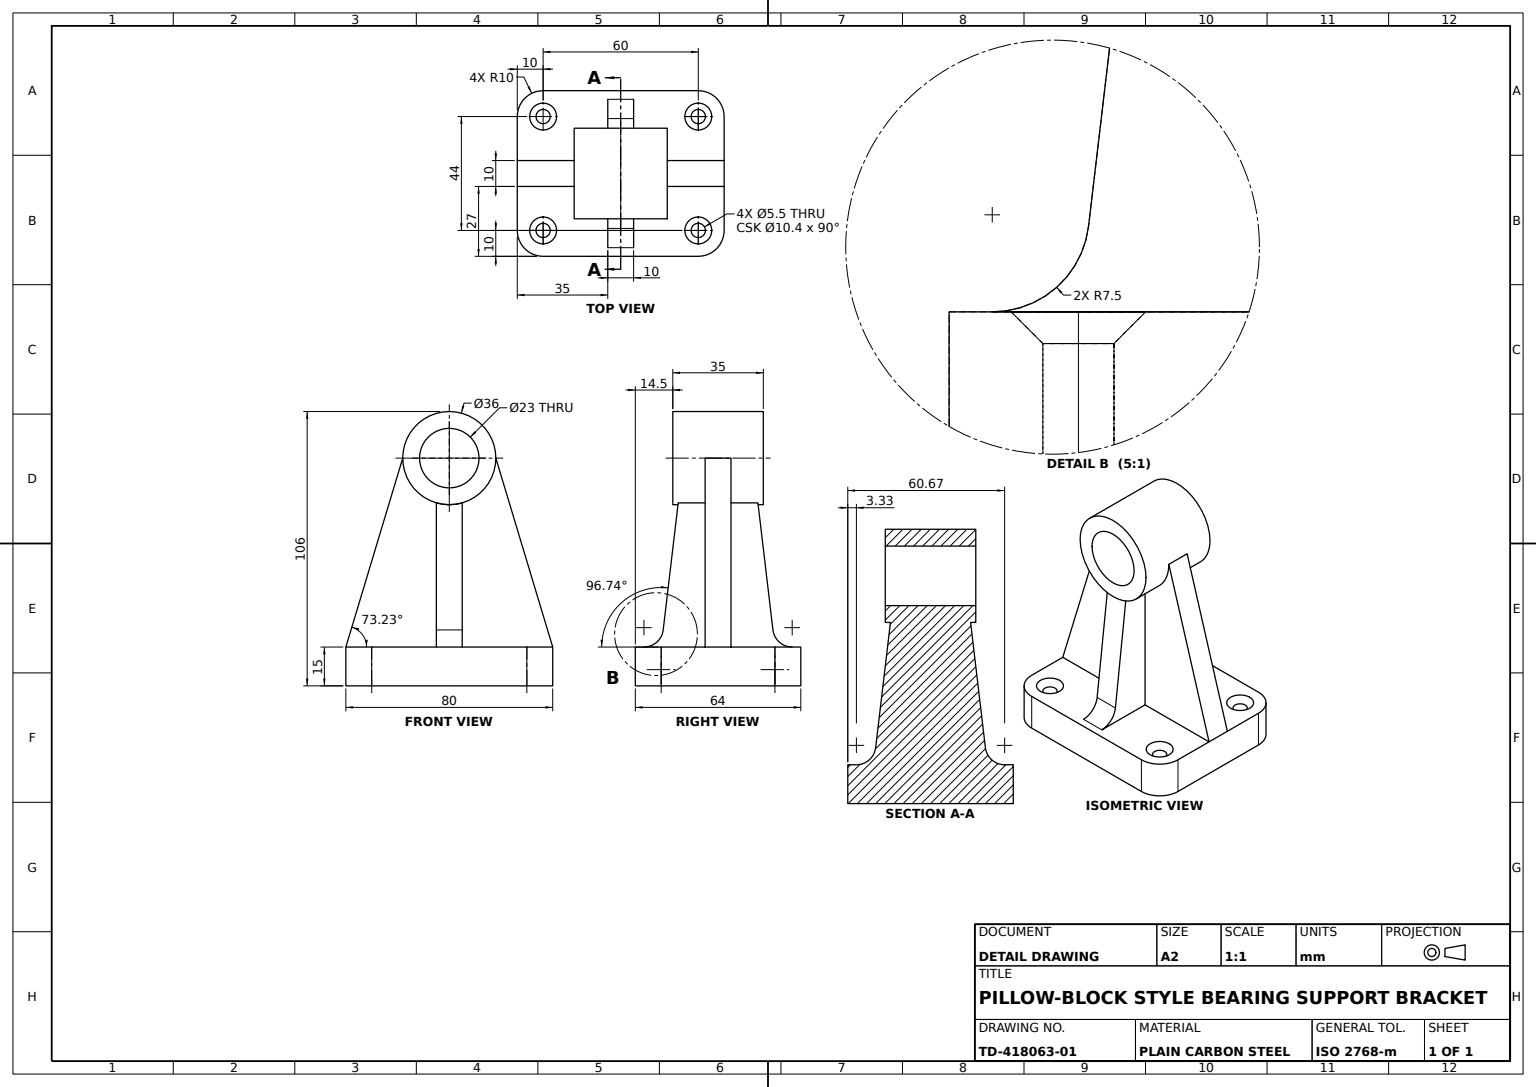
SolidWorks part; units mm, degrees
material "Plain Carbon Steel"
ref_plane "Front Plane" through (0, 0, 0) normal (0, 0, 1) x (1, 0, 0)
ref_plane "Top Plane" through (0, 0, 0) normal (0, 1, 0) x (1, 0, 0)
ref_plane "Right Plane" through (0, 0, 0) normal (1, 0, 0) x (0, 0, -1)
sketch "Base Plate Sketch" plane through (0, 0, 0) normal (0, 1, 0) x (1, 0, 0)
  line L1 (40, 0) -> (40, 22)
  line L2 (30, 32) -> (-30, 32)
  line L3 (-40, 22) -> (-40, -22)
  line L4 (-30, -32) -> (30, -32)
  line L5 (40, -22) -> (40, 0)
  arc A0 (-40, -22) -> (-30, -32) centre (-30, -22) ccw
  arc A1 (30, -32) -> (40, -22) centre (30, -22) ccw
  arc A2 (40, 22) -> (30, 32) centre (30, 22) ccw
  arc A3 (-30, 32) -> (-40, 22) centre (-30, 22) ccw
  point P8 (-40, -32)
  point P14 (40, 32)
  point P17 (-40, 32)
  dimension "D6" = 10
  dimension "D1" = 64
  dimension "D2" = 80
  dimension "D3" = 40
  dimension "D4" = 32
  dimension "D5" = 40
extrude "Base Plate" add sketch "Base Plate Sketch" along normal blind 15
sketch "Bearing Boss Sketch" plane through (0, 0, 0) normal (0, 0, 1) x (1, 0, 0)
  circle A0 centre (0, 88) radius 18
  circle A1 centre (0, 88) radius 11.5
  dimension "D1" = 36
  dimension "D3" = 23
  dimension "D2" = 88
extrude "Bearing Boss Ø36 Bore Ø23" add sketch "Bearing Boss Sketch" along normal mid plane 35 separate body
sketch "Upright Web Sketch" plane through (0, 0, 0) normal (0, 0, 1) x (1, 0, 0)
  line L0 (18, 88) -> (40, 15)
  line L1 (-18, 88) -> (-40, 15)
  line L2 (-40, 15) -> (40, 15)
  circle A0 centre (0, 88) radius 18 construction
  arc A1 (-18, 88) -> (18, 88) centre (0, 88) ccw
  dimension "D1" = 73
  dimension "D2" = 73
extrude "Upright Web" add sketch "Upright Web Sketch" along normal mid plane 10
hole_wizard "Mounting Holes M5 CSK" positions "Sketch4" profile "Sketch5" countersink size "M5" standard "ISO" end condition through all
sketch "Sketch4" plane through (0, 15, 0) normal (0, 1, 0) x (1, 0, 0)
  point P0 (-30, 22)
  point P3 (30, 22)
  point P6 (30, -22)
  point P9 (-30, -22)
sketch "Sketch5" plane through (-30, 15, -22) normal (1, 0, 0) x (0, 0, 1)
  line L0 (0, 0) -> (0, 15)
  line L1 (0, 15) -> (2.75, 15)
  line L2 (2.75, 15) -> (2.75, 2.45)
  line L3 (2.75, 2.45) -> (5.2, 0)
  line L5 (5.2, 0) -> (0, 0)
  line L6 (-2.75, 2.45) -> (-5.2, 0) construction
  line L11 (0, -6.35) -> (0, 107.95) construction
  dimension "Thru Hole Dia." = 5.5
  dimension "Thru Hole Depth" = 15
  dimension "Near C'Sink Dia." = 10.4
  dimension "Near C'Sink Angle" = 90
sketch "Support Rib Sketch" plane through (0, 0, 0) normal (1, 0, 0) x (0, 0, -1)
  line L2 (5, 70) -> (17.5, 70) construction
  line L3 (15.5, 70) -> (22, 15)
  dimension "D1" = 6.5
rib "Support Rib" sketch "Support Rib Sketch" sketch "Support Rib Sketch" thickness 10 extrusion direction parallel to sketch draft on no parameters "D1"=10
fillet "Rib Fillet R7.5" radius 7.5 1 edges at (0, 15, -22)
mirror "Support Rib Mirror" about plane through (0, 0, 0) normal (0, 0, 1) of "Rib Fillet R7.5", "Support Rib"
